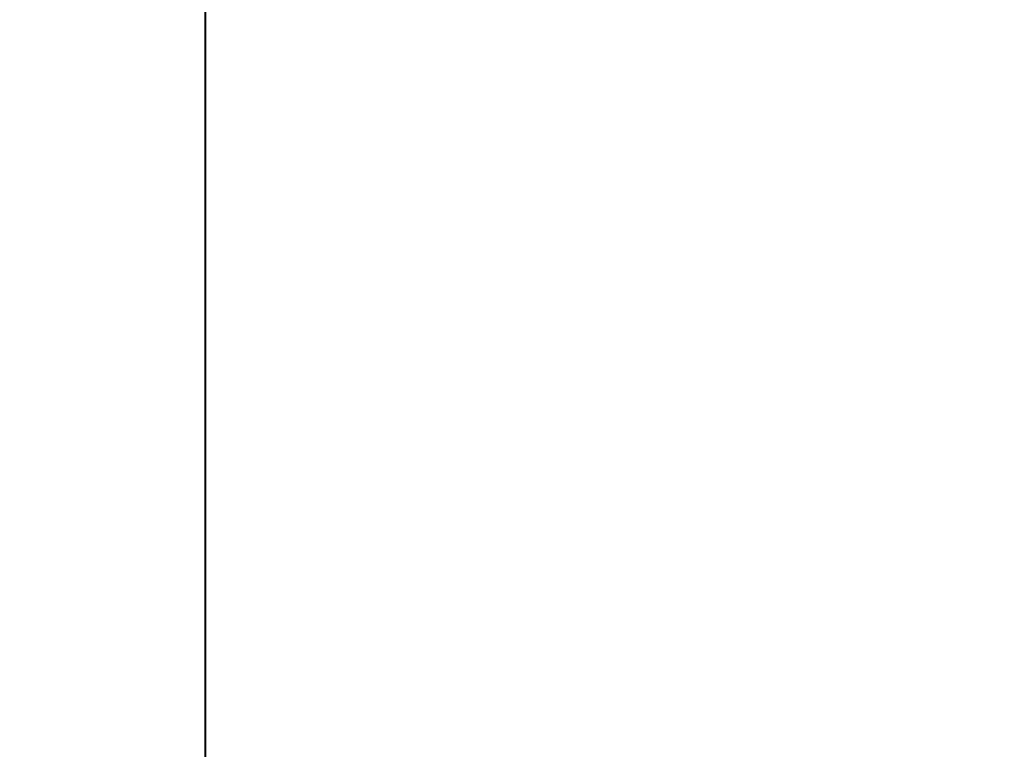
# Model space of a CAD drawing. Units: inches. Extents: x 459864 to 460310, y 324185 to 324787.
# Tile 85 of 112: x 460247.113242 to 460247.122182, y 324283.488802 to 324283.495429. Entities that reach past the tile are written whole.
import ezdxf

# ---------------------------------------------------------------- set-up
doc = ezdxf.new("R2010")
doc.units = ezdxf.units.IN
doc.layers.add('A-ANNO-DIMS', color=2, linetype='Continuous', lineweight=18)
doc.layers.add('A-WALL', color=7, linetype='Continuous', lineweight=40)
doc.styles.get("Standard").update_dxf_attribs({"font": 'arial.ttf'})
doc.dimstyles.new('ISO-25', dxfattribs={"dimtxt": 6, "dimasz": 2.5, "dimexe": 1.25, "dimexo": 0.625, "dimtad": 1, "dimdec": 1, "dimlunit": 3, "dimtxsty": 'Standard', "dimcen": 2.5, "dimadec": 0, "dimazin": 0, "dimtfac": 1, "dimtdec": 1, "dimtmove": 0, "dimatfit": 3, "dimfxl": 1, "dimarcsym": 0})

# ---------------------------------------------------------------- blocks, each defined once
blk = doc.blocks.new('*D21')
at = {"layer": 'A-ANNO-DIMS', "color": 0, "lineweight": -2, "transparency": 16777216}
for p, q in [((460247.7399266, 324715.4832328), (460309.5803685, 324715.4832328)), ((460308.3303685, 324712.9832328), (460308.3303685, 324285.9832328)), ((460247.7399266, 324283.4832328), (460309.5803685, 324283.4832328))]:
    blk.add_line(p, q, dxfattribs=at)
at = {"layer": 'A-ANNO-DIMS', "color": 0, "transparency": 16777216}
for points in [[(460307.9137019, 324712.9832328), (460308.7470352, 324712.9832328), (460308.3303685, 324715.4832328)], [(460307.9137019, 324285.9832328), (460308.7470352, 324285.9832328), (460308.3303685, 324283.4832328)]]:
    blk.add_solid(points, dxfattribs=at)
at = {"layer": 'Defpoints', "color": 0, "transparency": 16777216}
for p in [(460247.1149266, 324715.4832328), (460247.1149266, 324283.4832328), (460308.3303685, 324283.4832328)]:
    blk.add_point(p, dxfattribs=at)
at = {"layer": 'A-ANNO-DIMS', "color": 0, "transparency": 16777216, "insert": (460304.6398842, 324499.4832328), "char_height": 6, "attachment_point": 5, "rotation": 90}
blk.add_mtext("36'", dxfattribs=at)
blk = doc.blocks.new('*D62')
at = {"layer": 'A-ANNO-DIMS', "color": 0, "lineweight": -2, "transparency": 16777216}
for p, q in [((460247.739927, 324332.73872), (460278.764927, 324332.73872)), ((460277.514927, 324330.23872), (460277.514927, 324285.983233)), ((460247.739927, 324283.483233), (460278.764927, 324283.483233))]:
    blk.add_line(p, q, dxfattribs=at)
at = {"layer": 'A-ANNO-DIMS', "color": 0, "transparency": 16777216}
for points in [[(460277.0982603, 324330.23872), (460277.9315937, 324330.23872), (460277.514927, 324332.73872)], [(460277.0982603, 324285.983233), (460277.9315937, 324285.983233), (460277.514927, 324283.483233)]]:
    blk.add_solid(points, dxfattribs=at)
at = {"layer": 'Defpoints', "color": 0, "transparency": 16777216}
for p in [(460247.114927, 324332.73872), (460247.114927, 324283.483233), (460277.514927, 324283.483233)]:
    blk.add_point(p, dxfattribs=at)
at = {"layer": 'A-ANNO-DIMS', "color": 0, "transparency": 16777216, "insert": (460273.7876078, 324308.1109765), "char_height": 6, "attachment_point": 5, "rotation": 90}
blk.add_mtext('4\'-1 1/2"', dxfattribs=at)
blk = doc.blocks.new('*D67')
at = {"layer": 'A-ANNO-DIMS', "color": 0, "lineweight": -2, "transparency": 16777216}
for p, q in [((460208.114927, 324284.108233), (460208.114927, 324315.133233)), ((460247.114927, 324284.108233), (460247.114927, 324315.133233)), ((460210.614927, 324313.883233), (460244.614927, 324313.883233))]:
    blk.add_line(p, q, dxfattribs=at)
at = {"layer": 'A-ANNO-DIMS', "color": 0, "transparency": 16777216}
for points in [[(460210.614927, 324314.2998997), (460210.614927, 324313.4665663), (460208.114927, 324313.883233)], [(460244.614927, 324314.2998997), (460244.614927, 324313.4665663), (460247.114927, 324313.883233)]]:
    blk.add_solid(points, dxfattribs=at)
at = {"layer": 'Defpoints', "color": 0, "transparency": 16777216}
for p in [(460247.114927, 324313.883233), (460208.114927, 324283.483233), (460247.114927, 324283.483233)]:
    blk.add_point(p, dxfattribs=at)
at = {"layer": 'A-ANNO-DIMS', "color": 0, "transparency": 16777216, "insert": (460227.614927, 324317.5737173), "char_height": 6, "attachment_point": 5}
blk.add_mtext('3\'-3"', dxfattribs=at)

msp = doc.modelspace()

# ---------------------------------------------------------------- linework, layer by layer
at = {"layer": 'A-WALL'}
msp.add_line((460247.1149266, 324470.9832328), (460247.1149266, 324283.4832328), dxfattribs=at)

# ---------------------------------------------------------------- dimensions: what is measured, and where the dimension line sits
at = {"layer": 'A-ANNO-DIMS'}
for base, p1, p2, angle, override, picture, middle in [((460308.3303685, 324283.4832328), (460247.1149266, 324715.4832328), (460247.1149266, 324283.4832328), 90, {"dimclrd": 0, "dimclre": 0, "dimclrt": 0}, '*D21', (460304.6398842, 324499.4832328)), ((460277.514927, 324283.483233), (460247.114927, 324332.73872), (460247.114927, 324283.483233), 270, {"dimdec": 1, "dimlfac": 1, "dimrnd": 0, "dimzin": 1, "dimdsep": 46, "dimlunit": 4, "dimfrac": 2}, '*D62', (460273.7876078, 324308.1109765))]:
    dim = msp.add_linear_dim(base=base, p1=p1, p2=p2, angle=angle, dimstyle='ISO-25', override=override, dxfattribs=at)
    dim.commit()
    dim.dimension.update_dxf_attribs({"geometry": picture, "text_midpoint": middle})
dim = msp.add_linear_dim(base=(460247.114927, 324313.883233), p1=(460208.114927, 324283.483233), p2=(460247.114927, 324283.483233), dimstyle='ISO-25', override={"dimdec": 1, "dimlfac": 1, "dimrnd": 0, "dimzin": 1, "dimdsep": 46, "dimlunit": 4, "dimfrac": 2}, dxfattribs=at)
dim.commit()
dim.dimension.update_dxf_attribs({"geometry": '*D67', "text_midpoint": (460227.614927, 324317.5737173)})

doc.saveas('drawing.dxf')
